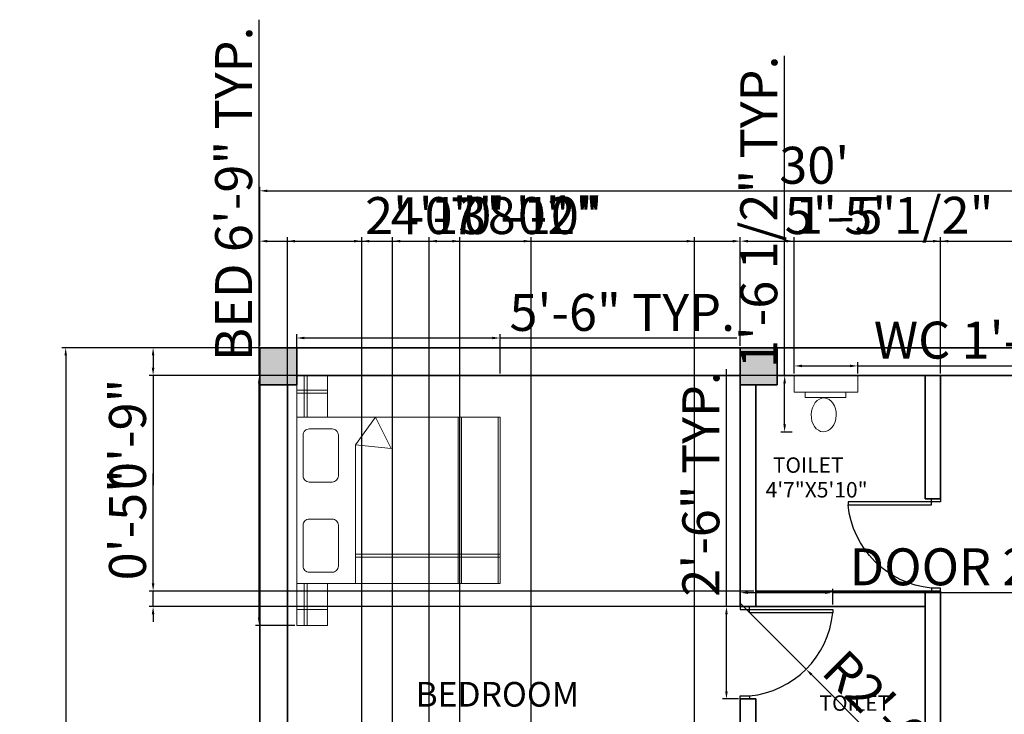
# Model space of a CAD drawing. Units: inches. Extents: x 2430 to 3058, y 1630 to 2396.
# Tile 3 of 4: x 2558 to 2878, y 2171 to 2396. Entities that reach past the tile are written whole.
import ezdxf

# ---------------------------------------------------------------- set-up
doc = ezdxf.new("R2010")
doc.units = ezdxf.units.IN
for name, color, linetype, lineweight in [('A-ANNO-DIMS', 7, 'Continuous', 18), ('A-AREA-IDEN', 131, 'Continuous', 18), ('A-COLS', 7, 'Continuous', 35), ('A-COLS-PATT', 1, 'Continuous', 13), ('A-DOOR', 40, 'Continuous', 25), ('A-FLOR-FIXT', 2, 'Continuous', 18), ('A-WALL', 7, 'Continuous', 35)]:
    doc.layers.add(name, color=color, linetype=linetype, lineweight=lineweight)
doc.layers.add('A-FURN', color=33, linetype='Continuous', lineweight=18, true_color=0xb0a07d)
doc.styles.get("Standard").update_dxf_attribs({"font": 'arial.ttf'})
doc.dimstyles.new('ISO-25', dxfattribs={"dimtxt": 12, "dimasz": 2.5, "dimexe": 1.25, "dimexo": 0.625, "dimtad": 1, "dimdec": 0, "dimlunit": 3, "dimtxsty": 'Standard', "dimcen": 2.5, "dimadec": 0, "dimazin": 0, "dimtfac": 1, "dimtdec": 0, "dimtmove": 0, "dimatfit": 3, "dimfxl": 1, "dimarcsym": 0})

# ---------------------------------------------------------------- blocks, each defined once
blk = doc.blocks.new('*D1')
at = {"layer": 'A-ANNO-DIMS', "color": 0, "lineweight": -2, "transparency": 16777216}
for p, q in [((2636, 2290.5), (2636, 2342.06)), ((2638.5, 2340.81), (2993.5, 2340.81)), ((2996, 2290.5), (2996, 2342.06))]:
    blk.add_line(p, q, dxfattribs=at)
at = {"layer": 'A-ANNO-DIMS', "color": 0, "transparency": 16777216}
for points in [[(2638.5, 2341.22), (2638.5, 2340.39), (2636, 2340.81)], [(2993.5, 2341.22), (2993.5, 2340.39), (2996, 2340.81)]]:
    blk.add_solid(points, dxfattribs=at)
at = {"layer": 'Defpoints', "color": 0, "transparency": 16777216}
for p in [(2996, 2340.81), (2636, 2289.88), (2996, 2289.88)]:
    blk.add_point(p, dxfattribs=at)
at = {"layer": 'A-ANNO-DIMS', "color": 0, "transparency": 16777216, "insert": (2816, 2347.56), "char_height": 12, "attachment_point": 5}
blk.add_mtext("30'", dxfattribs=at)
blk = doc.blocks.new('*D2')
at = {"layer": 'A-ANNO-DIMS', "color": 0, "lineweight": -2, "transparency": 16777216}
for p, q in [((2635.37, 2289.88), (2571.77, 2289.88)), ((2573.02, 2287.38), (2573.02, 1692.38)), ((2635.37, 1689.88), (2571.77, 1689.88))]:
    blk.add_line(p, q, dxfattribs=at)
at = {"layer": 'A-ANNO-DIMS', "color": 0, "transparency": 16777216}
for points in [[(2572.61, 2287.38), (2573.44, 2287.38), (2573.02, 2289.88)], [(2572.61, 1692.38), (2573.44, 1692.38), (2573.02, 1689.88)]]:
    blk.add_solid(points, dxfattribs=at)
at = {"layer": 'Defpoints', "color": 0, "transparency": 16777216}
for p in [(2636, 2289.88), (2573.02, 1689.88), (2636, 1689.88)]:
    blk.add_point(p, dxfattribs=at)
at = {"layer": 'A-ANNO-DIMS', "color": 0, "transparency": 16777216, "insert": (2566.27, 1989.88), "char_height": 12, "attachment_point": 5, "rotation": 90}
blk.add_mtext("50'", dxfattribs=at)
blk = doc.blocks.new('BED-DOUBLE')
for p, q in [((0, 67.56), (0, 81.12)), ((0, 81.12), (10, 81.12)), ((2.41, 67.56), (2.41, 81.12)), ((3.41, 67.56), (3.41, 81.12)), ((10, 81.12), (10, 67.56)), ((10, 76.33), (0, 76.33)), ((10, 75.33), (0, 75.33)), ((19.07, 58.56), (25.57, 67.56)), ((25.57, 67.56), (30.72, 57.43)), ((52.45, 67.56), (52.45, 13.56)), ((53.45, 67.56), (53.45, 13.56)), ((65.45, 67.56), (65.45, 13.56)), ((19.07, 13.56), (19.07, 58.56)), ((30.72, 57.43), (19.07, 58.56)), ((19.07, 23.13), (66, 23.13)), ((19.07, 22.13), (66, 22.13)), ((0, 0), (0, 13.56)), ((2.41, 0), (2.41, 13.56)), ((3.41, 0), (3.41, 13.56)), ((10, 13.56), (10, 0)), ((10, 6.18), (0, 6.18)), ((10, 5.18), (0, 5.18)), ((0, 0), (10, 0))]:
    blk.add_line(p, q)
blk.add_lwpolyline([(0, 67.56), (66, 67.56), (66, 13.56), (0, 13.56)], close=True)
for points in [[(4.09, 63.78), (11.52, 63.78, -0.414214), (13.52, 61.78), (13.52, 48.53, -0.414214), (11.52, 46.53), (4.09, 46.53, -0.414214), (2.09, 48.53), (2.09, 61.78, -0.414214)], [(4.09, 34.52), (11.52, 34.52, -0.414214), (13.52, 32.52), (13.52, 19.27, -0.414214), (11.52, 17.27), (4.09, 17.27, -0.414214), (2.09, 19.27), (2.09, 32.52, -0.414214)]]:
    blk.add_lwpolyline(points, format="xyb", close=True)
blk = doc.blocks.new('WC')
for points in [[(0, 18.29), (20.63, 18.29), (20.63, 12.83), (0, 12.83)], [(3.58, 12.83), (16.78, 12.83), (16.78, 11.1), (3.58, 11.1)]]:
    blk.add_lwpolyline(points, close=True)
blk.add_ellipse((9.59, 5.49), major_axis=(0.18, 5.49), ratio=0.738535)
blk = doc.blocks.new('DOOR-30')
for p, q in [((0, 30), (0, 29)), ((0, 29), (30, 29)), ((3, 28), (3, 30)), ((30, 29), (30, 28)), ((30, 28), (3, 28)), ((0, 0), (0, 1)), ((0, 1), (3, 1)), ((3, 1), (3, 0))]:
    blk.add_line(p, q)
blk.add_arc((0.14, 30.86), 30, 275.4764, 354.5236)
blk = doc.blocks.new('COL-12x12-EDGE')
for p, q in [((12, 12), (0, 12)), ((0, 12), (0, 0)), ((0, 0), (12, 0))]:
    blk.add_line(p, q)
blk = doc.blocks.new('*D15')
at = {"layer": 'A-ANNO-DIMS', "color": 0, "lineweight": -2, "transparency": 16777216}
for p, q in [((2635.83, 2280.88), (2635.83, 2396.37)), ((2647.37, 2280.88), (2634.58, 2280.88)), ((2635.83, 2202.26), (2635.83, 2278.38)), ((2647.37, 2199.76), (2634.58, 2199.76))]:
    blk.add_line(p, q, dxfattribs=at)
at = {"layer": 'A-ANNO-DIMS', "color": 0, "transparency": 16777216}
for points in [[(2635.41, 2278.38), (2636.24, 2278.38), (2635.83, 2280.88)], [(2635.41, 2202.26), (2636.24, 2202.26), (2635.83, 2199.76)]]:
    blk.add_solid(points, dxfattribs=at)
at = {"layer": 'Defpoints', "color": 0, "transparency": 16777216}
for p in [(2635.83, 2280.88), (2648, 2280.88), (2648, 2199.76)]:
    blk.add_point(p, dxfattribs=at)
at = {"layer": 'A-ANNO-DIMS', "color": 0, "transparency": 16777216, "insert": (2629.08, 2339.87), "char_height": 12, "attachment_point": 5, "rotation": 90}
blk.add_mtext('BED 6\'-9" TYP.', dxfattribs=at)
blk = doc.blocks.new('*D16')
at = {"layer": 'A-ANNO-DIMS', "color": 0, "lineweight": -2, "transparency": 16777216}
for p, q in [((2648, 2281.5), (2648, 2294.3)), ((2650.5, 2293.05), (2711.5, 2293.05)), ((2714, 2281.5), (2714, 2294.3)), ((2714, 2293.05), (2790.89, 2293.05))]:
    blk.add_line(p, q, dxfattribs=at)
at = {"layer": 'A-ANNO-DIMS', "color": 0, "transparency": 16777216}
for points in [[(2650.5, 2293.46), (2650.5, 2292.63), (2648, 2293.05)], [(2711.5, 2293.46), (2711.5, 2292.63), (2714, 2293.05)]]:
    blk.add_solid(points, dxfattribs=at)
at = {"layer": 'Defpoints', "color": 0, "transparency": 16777216}
for p in [(2714, 2293.05), (2648, 2280.88), (2714, 2280.88)]:
    blk.add_point(p, dxfattribs=at)
at = {"layer": 'A-ANNO-DIMS', "color": 0, "transparency": 16777216, "insert": (2753.69, 2299.8), "char_height": 12, "attachment_point": 5}
blk.add_mtext('5\'-6" TYP.', dxfattribs=at)
blk = doc.blocks.new('*D17')
at = {"layer": 'A-ANNO-DIMS', "color": 0, "lineweight": -2, "transparency": 16777216}
for p, q in [((2809.48, 2281.5), (2809.48, 2285.22)), ((2830.11, 2281.5), (2830.11, 2285.22)), ((2811.98, 2283.97), (2827.61, 2283.97)), ((2830.11, 2283.97), (2968.05, 2283.97))]:
    blk.add_line(p, q, dxfattribs=at)
at = {"layer": 'A-ANNO-DIMS', "color": 0, "transparency": 16777216}
for points in [[(2811.98, 2284.39), (2811.98, 2283.56), (2809.48, 2283.97)], [(2827.61, 2284.39), (2827.61, 2283.56), (2830.11, 2283.97)]]:
    blk.add_solid(points, dxfattribs=at)
at = {"layer": 'Defpoints', "color": 0, "transparency": 16777216}
for p in [(2830.11, 2283.97), (2809.48, 2280.88), (2830.11, 2280.88)]:
    blk.add_point(p, dxfattribs=at)
at = {"layer": 'A-ANNO-DIMS', "color": 0, "transparency": 16777216, "insert": (2900.33, 2290.8), "char_height": 12, "attachment_point": 5}
blk.add_mtext('WC 1\'-8 1/2" TYP.', dxfattribs=at)
blk = doc.blocks.new('*D18')
at = {"layer": 'A-ANNO-DIMS', "color": 0, "lineweight": -2, "transparency": 16777216}
for p, q in [((2806.38, 2280.88), (2806.38, 2384.61)), ((2808.85, 2280.88), (2805.13, 2280.88)), ((2806.38, 2265.02), (2806.38, 2278.38)), ((2808.85, 2262.52), (2805.13, 2262.52))]:
    blk.add_line(p, q, dxfattribs=at)
at = {"layer": 'A-ANNO-DIMS', "color": 0, "transparency": 16777216}
for points in [[(2805.97, 2278.38), (2806.8, 2278.38), (2806.38, 2280.88)], [(2805.97, 2265.02), (2806.8, 2265.02), (2806.38, 2262.52)]]:
    blk.add_solid(points, dxfattribs=at)
at = {"layer": 'Defpoints', "color": 0, "transparency": 16777216}
for p in [(2806.38, 2280.88), (2809.48, 2280.88), (2809.48, 2262.52)]:
    blk.add_point(p, dxfattribs=at)
at = {"layer": 'A-ANNO-DIMS', "color": 0, "transparency": 16777216, "insert": (2799.55, 2333.99), "char_height": 12, "attachment_point": 5, "rotation": 90}
blk.add_mtext('1\'-6 1/2" TYP.', dxfattribs=at)
blk = doc.blocks.new('*D21')
at = {"layer": 'A-ANNO-DIMS', "color": 0, "lineweight": -2, "transparency": 16777216}
for p, q in [((2792, 2206.5), (2792, 2211.63)), ((2822, 2206.5), (2822, 2211.63)), ((2794.5, 2210.38), (2819.5, 2210.38)), ((2822, 2210.38), (2953.24, 2210.38))]:
    blk.add_line(p, q, dxfattribs=at)
at = {"layer": 'A-ANNO-DIMS', "color": 0, "transparency": 16777216}
for points in [[(2794.5, 2210.79), (2794.5, 2209.96), (2792, 2210.38)], [(2819.5, 2210.79), (2819.5, 2209.96), (2822, 2210.38)]]:
    blk.add_solid(points, dxfattribs=at)
at = {"layer": 'Defpoints', "color": 0, "transparency": 16777216}
for p in [(2822, 2210.38), (2792, 2205.88), (2822, 2205.88)]:
    blk.add_point(p, dxfattribs=at)
at = {"layer": 'A-ANNO-DIMS', "color": 0, "transparency": 16777216, "insert": (2888.87, 2217.21), "char_height": 12, "attachment_point": 5}
blk.add_mtext('DOOR 2\'-6" TYP.', dxfattribs=at)
blk = doc.blocks.new('*D22')
at = {"layer": 'A-ANNO-DIMS', "color": 0, "lineweight": -2, "transparency": 16777216}
for p, q in [((2787.5, 2205.88), (2787.5, 2282.98)), ((2791.37, 2205.88), (2786.25, 2205.88)), ((2787.5, 2178.38), (2787.5, 2203.38)), ((2791.37, 2175.88), (2786.25, 2175.88))]:
    blk.add_line(p, q, dxfattribs=at)
at = {"layer": 'A-ANNO-DIMS', "color": 0, "transparency": 16777216}
for points in [[(2787.08, 2203.38), (2787.91, 2203.38), (2787.5, 2205.88)], [(2787.08, 2178.38), (2787.91, 2178.38), (2787.5, 2175.88)]]:
    blk.add_solid(points, dxfattribs=at)
at = {"layer": 'Defpoints', "color": 0, "transparency": 16777216}
for p in [(2787.5, 2205.88), (2792, 2205.88), (2792, 2175.88)]:
    blk.add_point(p, dxfattribs=at)
at = {"layer": 'A-ANNO-DIMS', "color": 0, "transparency": 16777216, "insert": (2780.74, 2245.68), "char_height": 12, "attachment_point": 5, "rotation": 90}
blk.add_mtext('2\'-6" TYP.', dxfattribs=at)
blk = doc.blocks.new('*D27')
at = {"layer": 'A-ANNO-DIMS', "color": 0, "lineweight": -2, "transparency": 16777216}
for p, q in [((2636, 2290.5), (2636, 2325.73)), ((2638.5, 2324.48), (2789.5, 2324.48)), ((2792, 2290.5), (2792, 2325.73))]:
    blk.add_line(p, q, dxfattribs=at)
at = {"layer": 'A-ANNO-DIMS', "color": 0, "transparency": 16777216}
for points in [[(2638.5, 2324.89), (2638.5, 2324.06), (2636, 2324.48)], [(2789.5, 2324.89), (2789.5, 2324.06), (2792, 2324.48)]]:
    blk.add_solid(points, dxfattribs=at)
at = {"layer": 'Defpoints', "color": 0, "transparency": 16777216}
for p in [(2792, 2324.48), (2636, 2289.88), (2792, 2289.88)]:
    blk.add_point(p, dxfattribs=at)
at = {"layer": 'A-ANNO-DIMS', "color": 0, "transparency": 16777216, "insert": (2714, 2331.23), "char_height": 12, "attachment_point": 5}
blk.add_mtext('13\'-0"', dxfattribs=at)
blk = doc.blocks.new('*D28')
at = {"layer": 'A-ANNO-DIMS', "color": 0, "lineweight": -2, "transparency": 16777216}
for p, q in [((2792, 2290.5), (2792, 2325.73)), ((2794.5, 2324.48), (2854.5, 2324.48)), ((2857, 2281.5), (2857, 2325.73))]:
    blk.add_line(p, q, dxfattribs=at)
at = {"layer": 'A-ANNO-DIMS', "color": 0, "transparency": 16777216}
for points in [[(2794.5, 2324.89), (2794.5, 2324.06), (2792, 2324.48)], [(2854.5, 2324.89), (2854.5, 2324.06), (2857, 2324.48)]]:
    blk.add_solid(points, dxfattribs=at)
at = {"layer": 'Defpoints', "color": 0, "transparency": 16777216}
for p in [(2857, 2324.48), (2792, 2289.88), (2857, 2280.88)]:
    blk.add_point(p, dxfattribs=at)
at = {"layer": 'A-ANNO-DIMS', "color": 0, "transparency": 16777216, "insert": (2824.5, 2331.21), "char_height": 12, "attachment_point": 5}
blk.add_mtext('5\'-5"', dxfattribs=at)
blk = doc.blocks.new('*D29')
at = {"layer": 'A-ANNO-DIMS', "color": 0, "lineweight": -2, "transparency": 16777216}
for p, q in [((2857, 2281.5), (2857, 2325.73)), ((2859.5, 2324.48), (2993.5, 2324.48)), ((2996, 2290.5), (2996, 2325.73))]:
    blk.add_line(p, q, dxfattribs=at)
at = {"layer": 'A-ANNO-DIMS', "color": 0, "transparency": 16777216}
for points in [[(2859.5, 2324.89), (2859.5, 2324.06), (2857, 2324.48)], [(2993.5, 2324.89), (2993.5, 2324.06), (2996, 2324.48)]]:
    blk.add_solid(points, dxfattribs=at)
at = {"layer": 'Defpoints', "color": 0, "transparency": 16777216}
for p in [(2996, 2324.48), (2996, 2289.88), (2857, 2280.88)]:
    blk.add_point(p, dxfattribs=at)
at = {"layer": 'A-ANNO-DIMS', "color": 0, "transparency": 16777216, "insert": (2926.5, 2331.13), "char_height": 12, "attachment_point": 5}
blk.add_mtext('11\'-7"', dxfattribs=at)
blk = doc.blocks.new('*D44')
at = {"layer": 'A-ANNO-DIMS', "color": 0, "lineweight": -2, "transparency": 16777216}
for p, q in [((2691, 1913.5), (2691, 2325.73)), ((2693.5, 2324.48), (2698.5, 2324.48)), ((2701, 1913.5), (2701, 2325.73)), ((2701, 2324.48), (2745.97, 2324.48))]:
    blk.add_line(p, q, dxfattribs=at)
at = {"layer": 'A-ANNO-DIMS', "color": 0, "transparency": 16777216}
for points in [[(2693.5, 2324.89), (2693.5, 2324.06), (2691, 2324.48)], [(2698.5, 2324.89), (2698.5, 2324.06), (2701, 2324.48)]]:
    blk.add_solid(points, dxfattribs=at)
at = {"layer": 'Defpoints', "color": 0, "transparency": 16777216}
for p in [(2701, 2324.48), (2691, 1912.88), (2701, 1912.88)]:
    blk.add_point(p, dxfattribs=at)
at = {"layer": 'A-ANNO-DIMS', "color": 0, "transparency": 16777216, "insert": (2724.73, 2331.23), "char_height": 12, "attachment_point": 5}
blk.add_mtext('0\'-10"', dxfattribs=at)
blk = doc.blocks.new('*D46')
at = {"layer": 'A-ANNO-DIMS', "color": 0, "lineweight": -2, "transparency": 16777216}
for p, q in [((2601.4, 2213.38), (2601.4, 2249.03)), ((2796.37, 2210.88), (2600.15, 2210.88)), ((2601.4, 2205.88), (2601.4, 2210.88)), ((2796.37, 2205.88), (2600.15, 2205.88)), ((2601.4, 2203.38), (2601.4, 2200.88))]:
    blk.add_line(p, q, dxfattribs=at)
at = {"layer": 'A-ANNO-DIMS', "color": 0, "transparency": 16777216}
for points in [[(2600.98, 2213.38), (2601.81, 2213.38), (2601.4, 2210.88)], [(2600.98, 2203.38), (2601.81, 2203.38), (2601.4, 2205.88)]]:
    blk.add_solid(points, dxfattribs=at)
at = {"layer": 'Defpoints', "color": 0, "transparency": 16777216}
for p in [(2601.4, 2210.88), (2797, 2210.88), (2797, 2205.88)]:
    blk.add_point(p, dxfattribs=at)
at = {"layer": 'A-ANNO-DIMS', "color": 0, "transparency": 16777216, "insert": (2594.64, 2232.45), "char_height": 12, "attachment_point": 5, "rotation": 90}
blk.add_mtext('0\'-5"', dxfattribs=at)
blk = doc.blocks.new('*D47')
at = {"layer": 'A-ANNO-DIMS', "color": 0, "lineweight": -2, "transparency": 16777216}
for p, q in [((2792, 2290.5), (2792, 2325.73)), ((2794.5, 2324.48), (2806.98, 2324.48)), ((2809.48, 2281.5), (2809.48, 2325.73)), ((2809.48, 2324.48), (2871.96, 2324.48))]:
    blk.add_line(p, q, dxfattribs=at)
at = {"layer": 'A-ANNO-DIMS', "color": 0, "transparency": 16777216}
for points in [[(2794.5, 2324.89), (2794.5, 2324.06), (2792, 2324.48)], [(2806.98, 2324.89), (2806.98, 2324.06), (2809.48, 2324.48)]]:
    blk.add_solid(points, dxfattribs=at)
at = {"layer": 'Defpoints', "color": 0, "transparency": 16777216}
for p in [(2809.48, 2324.48), (2792, 2289.88), (2809.48, 2280.88)]:
    blk.add_point(p, dxfattribs=at)
at = {"layer": 'A-ANNO-DIMS', "color": 0, "transparency": 16777216, "insert": (2841.97, 2331.31), "char_height": 12, "attachment_point": 5}
blk.add_mtext('1\'-5 1/2"', dxfattribs=at)
blk = doc.blocks.new('*D48')
at = {"layer": 'A-ANNO-DIMS', "color": 0, "lineweight": -2, "transparency": 16777216}
for p, q in [((2791.37, 2289.88), (2600.15, 2289.88)), ((2601.4, 2287.38), (2601.4, 2283.38)), ((2808.85, 2280.88), (2600.15, 2280.88)), ((2601.4, 2280.88), (2601.4, 2245.23))]:
    blk.add_line(p, q, dxfattribs=at)
at = {"layer": 'A-ANNO-DIMS', "color": 0, "transparency": 16777216}
for points in [[(2600.98, 2287.38), (2601.81, 2287.38), (2601.4, 2289.88)], [(2600.98, 2283.38), (2601.81, 2283.38), (2601.4, 2280.88)]]:
    blk.add_solid(points, dxfattribs=at)
at = {"layer": 'Defpoints', "color": 0, "transparency": 16777216}
for p in [(2792, 2289.88), (2601.4, 2280.88), (2809.48, 2280.88)]:
    blk.add_point(p, dxfattribs=at)
at = {"layer": 'A-ANNO-DIMS', "color": 0, "transparency": 16777216, "insert": (2594.64, 2261.8), "char_height": 12, "attachment_point": 5, "rotation": 90}
blk.add_mtext('0\'-9"', dxfattribs=at)
blk = doc.blocks.new('*D58')
at = {"layer": 'A-ANNO-DIMS', "color": 0, "lineweight": -2, "transparency": 16777216}
for p, q in [((2669.13, 2100.28), (2669.13, 2325.73)), ((2671.63, 2324.48), (2721.64, 2324.48)), ((2724.14, 2100.28), (2724.14, 2325.73))]:
    blk.add_line(p, q, dxfattribs=at)
at = {"layer": 'A-ANNO-DIMS', "color": 0, "transparency": 16777216}
for points in [[(2671.63, 2324.89), (2671.63, 2324.06), (2669.13, 2324.48)], [(2721.64, 2324.89), (2721.64, 2324.06), (2724.14, 2324.48)]]:
    blk.add_solid(points, dxfattribs=at)
at = {"layer": 'Defpoints', "color": 0, "transparency": 16777216}
for p in [(2724.14, 2324.48), (2669.13, 2099.65), (2724.14, 2099.65)]:
    blk.add_point(p, dxfattribs=at)
at = {"layer": 'A-ANNO-DIMS', "color": 0, "transparency": 16777216, "insert": (2696.63, 2331.1), "char_height": 12, "attachment_point": 5}
blk.add_mtext('4\'-7"', dxfattribs=at)
blk = doc.blocks.new('*D60')
at = {"layer": 'A-ANNO-DIMS', "color": 0, "lineweight": -2, "transparency": 16777216}
for p, q in [((2679.11, 2038.23), (2679.11, 2325.73)), ((2681.61, 2324.48), (2774.61, 2324.48)), ((2777.11, 2038.23), (2777.11, 2325.73))]:
    blk.add_line(p, q, dxfattribs=at)
at = {"layer": 'A-ANNO-DIMS', "color": 0, "transparency": 16777216}
for points in [[(2681.61, 2324.89), (2681.61, 2324.06), (2679.11, 2324.48)], [(2774.61, 2324.89), (2774.61, 2324.06), (2777.11, 2324.48)]]:
    blk.add_solid(points, dxfattribs=at)
at = {"layer": 'Defpoints', "color": 0, "transparency": 16777216}
for p in [(2777.11, 2324.48), (2679.11, 2037.6), (2777.11, 2037.6)]:
    blk.add_point(p, dxfattribs=at)
at = {"layer": 'A-ANNO-DIMS', "color": 0, "transparency": 16777216, "insert": (2728.11, 2331.23), "char_height": 12, "attachment_point": 5}
blk.add_mtext('8\'-2"', dxfattribs=at)
blk = doc.blocks.new('*D63')
at = {"layer": 'A-ANNO-DIMS', "color": 0, "lineweight": -2, "transparency": 16777216}
for p, q in [((2645, 2002.5), (2645, 2325.73)), ((2647.5, 2324.48), (2666.63, 2324.48)), ((2669.13, 2073.52), (2669.13, 2325.73)), ((2669.13, 2324.48), (2704.98, 2324.48))]:
    blk.add_line(p, q, dxfattribs=at)
at = {"layer": 'A-ANNO-DIMS', "color": 0, "transparency": 16777216}
for points in [[(2647.5, 2324.89), (2647.5, 2324.06), (2645, 2324.48)], [(2666.63, 2324.89), (2666.63, 2324.06), (2669.13, 2324.48)]]:
    blk.add_solid(points, dxfattribs=at)
at = {"layer": 'Defpoints', "color": 0, "transparency": 16777216}
for p in [(2669.13, 2324.48), (2669.13, 2072.9), (2645, 2001.88)]:
    blk.add_point(p, dxfattribs=at)
at = {"layer": 'A-ANNO-DIMS', "color": 0, "transparency": 16777216, "insert": (2688.3, 2331.23), "char_height": 12, "attachment_point": 5}
blk.add_mtext('2\'-0"', dxfattribs=at)
blk = doc.blocks.new('*D68')
at = {"layer": 'A-ANNO-DIMS', "color": 0, "lineweight": -2, "transparency": 16777216}
for p, q in [((2792.13, 2206.74), (2813.35, 2185.53)), ((2848.44, 2150.43), (2815.11, 2183.76))]:
    blk.add_line(p, q, dxfattribs=at)
at = {"layer": 'A-ANNO-DIMS', "color": 0, "transparency": 16777216}
blk.add_solid([(2815.41, 2184.05), (2814.82, 2183.47), (2813.35, 2185.53)], dxfattribs=at)
at = {"layer": 'Defpoints', "color": 0, "transparency": 16777216}
for p in [(2792.13, 2206.74), (2813.35, 2185.53)]:
    blk.add_point(p, dxfattribs=at)
at = {"layer": 'A-ANNO-DIMS', "color": 0, "transparency": 16777216, "insert": (2837.44, 2170.99), "char_height": 12, "attachment_point": 5, "rotation": 315.0012}
blk.add_mtext('R2\'-6"', dxfattribs=at)

msp = doc.modelspace()

# ---------------------------------------------------------------- hatches: boundary and pattern name
at = {"layer": 'A-COLS-PATT'}
h = msp.add_hatch(color=256, dxfattribs=at)
h.dxf.hatch_style = 1
h.paths.add_polyline_path([(2648, 2289.88), (2636, 2289.88), (2636, 2277.88), (2648, 2277.88), (2648, 2280.88)])
h = msp.add_hatch(color=256, dxfattribs=at)
h.dxf.hatch_style = 1
h.paths.add_polyline_path([(2804, 2289.88), (2792, 2289.88), (2792, 2280.88), (2792, 2277.88), (2804, 2277.88)])

# ---------------------------------------------------------------- linework, layer by layer
at = {"layer": 'A-COLS'}
for p, q in [((2792, 2280.88), (2792, 2289.88)), ((2804, 2277.88), (2804, 2289.88)), ((2792, 2277.88), (2804, 2277.88))]:
    msp.add_line(p, q, dxfattribs=at)
at = {"layer": 'A-WALL'}
for p, q in [((2648, 2280.88), (2792, 2280.88)), ((2792, 2205.88), (2792, 2280.88)), ((2804, 2280.88), (2984, 2280.88)), ((2852, 2240.88), (2852, 2280.88)), ((2857, 2240.88), (2857, 2280.88)), ((2645, 2133.88), (2645, 2277.88)), ((2797, 2205.88), (2797, 2277.88)), ((2852, 2240.88), (2857, 2240.88)), ((2797, 2210.88), (2857, 2210.88)), ((2852, 2130.88), (2852, 2210.88)), ((2857, 2121.88), (2857, 2210.88)), ((2792, 2205.88), (2852, 2205.88)), ((2792, 2175.88), (2797, 2175.88)), ((2792, 2121.88), (2792, 2175.88)), ((2797, 2133.88), (2797, 2175.88))]:
    msp.add_line(p, q, dxfattribs=at)
msp.add_lwpolyline([(2636, 2289.88), (2996, 2289.88), (2996, 1689.88), (2636, 1689.88)], close=True, dxfattribs=at)

# ---------------------------------------------------------------- block references
at = {"layer": 'A-COLS', "rotation": 180}
msp.add_blockref('COL-12x12-EDGE', (2648, 2289.88), dxfattribs=at)
at = {"layer": 'A-DOOR', "extrusion": (0, 0, -1), "zscale": -1}
msp.add_blockref('DOOR-30', (-2857, 2210.88), dxfattribs=at)
at = {"layer": 'A-DOOR'}
msp.add_blockref('DOOR-30', (2792, 2175.88), dxfattribs=at)
at = {"layer": 'A-FLOR-FIXT'}
msp.add_blockref('WC', (2809.48, 2262.59), dxfattribs=at)
at = {"layer": 'A-FURN'}
msp.add_blockref('BED-DOUBLE', (2648, 2199.76), dxfattribs=at)

# ---------------------------------------------------------------- texts
at = {"layer": 'A-AREA-IDEN'}
for tag, p, height in [('TOILET', (2802.56, 2249.29), 5), ('4\'7"X5\'10"', (2800.21, 2241.27), 5), ('BEDROOM', (2686.58, 2173.39), 8), ('TOILET', (2817.68, 2172.02), 5)]:
    msp.add_attdef(tag, p, '', height=height, dxfattribs=at)

# ---------------------------------------------------------------- dimensions: what is measured, and where the dimension line sits
at = {"layer": 'A-ANNO-DIMS'}
for base, p1, p2, text, picture, middle in [((2635.83, 2280.88), (2648, 2199.76), (2648, 2280.88), 'BED <> TYP.', '*D15', (2629.08, 2339.87)), ((2806.38, 2280.88), (2809.48, 2262.52), (2809.48, 2280.88), '<> TYP.', '*D18', (2799.55, 2333.99)), ((2787.5, 2205.88), (2792, 2175.88), (2792, 2205.88), '<> TYP.', '*D22', (2780.74, 2245.68))]:
    dim = msp.add_linear_dim(base=base, p1=p1, p2=p2, angle=90, text=text, dimstyle='ISO-25', override={"dimdec": 1, "dimlfac": 1, "dimrnd": 0, "dimzin": 1, "dimdsep": 46, "dimlunit": 4, "dimfrac": 2}, dxfattribs=at)
    dim.commit()
    dim.dimension.update_dxf_attribs({"geometry": picture, "text_midpoint": middle})
for base, p1, p2, override, picture, middle in [((2996, 2340.81), (2636, 2289.88), (2996, 2289.88), {"dimclrd": 0, "dimclre": 0, "dimclrt": 0}, '*D1', (2816, 2347.56)), ((2809.48, 2324.48), (2792, 2289.88), (2809.48, 2280.88), {"dimdec": 1, "dimlfac": 1, "dimrnd": 0, "dimzin": 1, "dimdsep": 46, "dimlunit": 4, "dimfrac": 2}, '*D47', (2841.97, 2331.31)), ((2792, 2324.48), (2636, 2289.88), (2792, 2289.88), {"dimdec": 1, "dimlfac": 1, "dimrnd": 0, "dimzin": 1, "dimdsep": 46, "dimlunit": 4, "dimfrac": 2}, '*D27', (2714, 2331.23)), ((2669.13, 2324.48), (2645, 2001.88), (2669.13, 2072.9), {"dimdec": 1, "dimlfac": 1, "dimrnd": 0, "dimzin": 1, "dimdsep": 46, "dimlunit": 4, "dimfrac": 2}, '*D63', (2688.3, 2331.23)), ((2777.11, 2324.48), (2679.11, 2037.6), (2777.11, 2037.6), {"dimdec": 1, "dimlfac": 1, "dimrnd": 0, "dimzin": 1, "dimdsep": 46, "dimlunit": 4, "dimfrac": 2}, '*D60', (2728.11, 2331.23)), ((2701, 2324.48), (2691, 1912.88), (2701, 1912.88), {"dimdec": 1, "dimlfac": 1, "dimrnd": 0, "dimzin": 1, "dimdsep": 46, "dimlunit": 4, "dimfrac": 2}, '*D44', (2724.73, 2331.23)), ((2724.14, 2324.48), (2669.13, 2099.65), (2724.14, 2099.65), {"dimdec": 1, "dimlfac": 1, "dimrnd": 0, "dimzin": 1, "dimdsep": 46, "dimlunit": 4, "dimfrac": 2}, '*D58', (2696.63, 2331.1)), ((2857, 2324.48), (2792, 2289.88), (2857, 2280.88), {"dimdec": 1, "dimlfac": 1, "dimrnd": 0, "dimzin": 1, "dimdsep": 46, "dimlunit": 4, "dimfrac": 2}, '*D28', (2824.5, 2331.21)), ((2996, 2324.48), (2857, 2280.88), (2996, 2289.88), {"dimdec": 1, "dimlfac": 1, "dimrnd": 0, "dimzin": 1, "dimdsep": 46, "dimlunit": 4, "dimfrac": 2}, '*D29', (2926.5, 2331.13))]:
    dim = msp.add_linear_dim(base=base, p1=p1, p2=p2, dimstyle='ISO-25', override=override, dxfattribs=at)
    dim.commit()
    dim.dimension.update_dxf_attribs({"geometry": picture, "text_midpoint": middle})
for base, p1, p2, text, picture, middle in [((2830.11, 2283.97), (2809.48, 2280.88), (2830.11, 2280.88), 'WC <> TYP.', '*D17', (2900.33, 2290.8)), ((2714, 2293.05), (2648, 2280.88), (2714, 2280.88), '<> TYP.', '*D16', (2753.69, 2299.8)), ((2822, 2210.38), (2792, 2205.88), (2822, 2205.88), 'DOOR <> TYP.', '*D21', (2888.87, 2217.21))]:
    dim = msp.add_linear_dim(base=base, p1=p1, p2=p2, text=text, dimstyle='ISO-25', override={"dimdec": 1, "dimlfac": 1, "dimrnd": 0, "dimzin": 1, "dimdsep": 46, "dimlunit": 4, "dimfrac": 2}, dxfattribs=at)
    dim.commit()
    dim.dimension.update_dxf_attribs({"geometry": picture, "text_midpoint": middle})
for base, p1, p2, override, picture, middle in [((2573.02, 1689.88), (2636, 2289.88), (2636, 1689.88), {"dimclrd": 0, "dimclre": 0, "dimclrt": 0}, '*D2', (2566.27, 1989.88)), ((2601.4, 2280.88), (2792, 2289.88), (2809.48, 2280.88), {"dimdec": 1, "dimlfac": 1, "dimrnd": 0, "dimzin": 1, "dimdsep": 46, "dimlunit": 4, "dimfrac": 2}, '*D48', (2594.64, 2261.8)), ((2601.4, 2210.88), (2797, 2205.88), (2797, 2210.88), {"dimdec": 1, "dimlfac": 1, "dimrnd": 0, "dimzin": 1, "dimdsep": 46, "dimlunit": 4, "dimfrac": 2}, '*D46', (2594.64, 2232.45))]:
    dim = msp.add_linear_dim(base=base, p1=p1, p2=p2, angle=90, dimstyle='ISO-25', override=override, dxfattribs=at)
    dim.commit()
    dim.dimension.update_dxf_attribs({"geometry": picture, "text_midpoint": middle})
dim = msp.add_radius_dim(center=(2792.13, 2206.74), mpoint=(2813.35, 2185.53), dimstyle='ISO-25', override={"dimdec": 1, "dimlfac": 1, "dimrnd": 0, "dimzin": 1, "dimdsep": 46, "dimlunit": 4, "dimfrac": 2}, dxfattribs=at)
dim.commit()
dim.dimension.update_dxf_attribs({"geometry": '*D68', "text_midpoint": (2837.44, 2170.99)})

doc.saveas('drawing.dxf')
